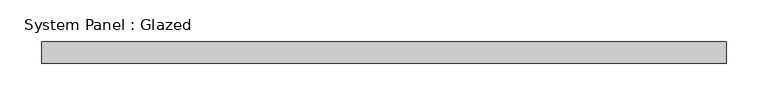
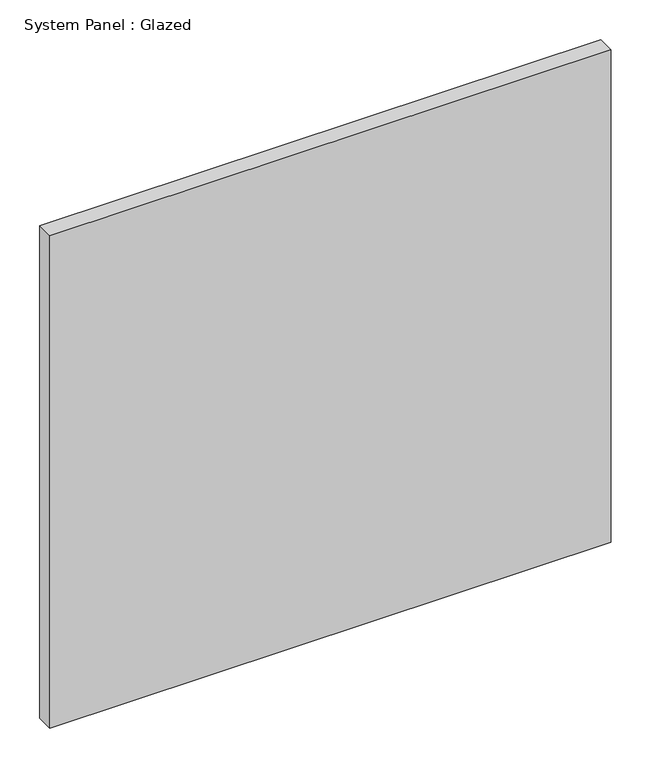
"""IFC4 building model written with IfcOpenShell, lengths in millimetres: plate geometry, System Panel : Glazed."""

from ifc_helpers import new_model, si_unit, origin, origin_with_axes, place, context, project, spatial, polyline, outline, extrude, source, transform, mapped, element, save


def system_panel_glazed_8adc4deb(model_context):
    return source(origin(), model_context, "Body", "SweptSolid", [
        extrude(outline(polyline([(409.575, 19.05), (-409.575, 19.05), (-409.575, 44.45), (409.575, 44.45), (409.575, 19.05)])), origin_with_axes(), (0.0, 0.0, 1.0), 759.593224),
    ])


if __name__ == "__main__":
    model = new_model("IFC4")
    model_context = context("Model", 3, world=origin())
    ifc_project = project(units=[si_unit("LENGTHUNIT", "METRE", prefix="MILLI")], contexts=[model_context])
    site = spatial("IfcSite", under=ifc_project)
    building = spatial("IfcBuilding", under=site)
    placement = place(None, origin())
    system_panel_glazed_shape = system_panel_glazed_8adc4deb(model_context)
    element("IfcPlate", 1, ObjectType="System Panel : Glazed", at=placement, inside=building, context=model_context, shape_type="MappedRepresentation", body=[
        mapped(system_panel_glazed_shape, transform((0.0, 0.0, 0.0), x_axis=(1.0, 0.0, 0.0), y_axis=(0.0, 1.0, 0.0), z_axis=(0.0, 0.0, 1.0))),
    ])
    save(model, "model.ifc")

# Revit data of these elements
# Type "System Panel : Glazed"
#   Construction Type Id = "GSP4R"
#   Analytic Construction = "1/8 in Pilkington single glazing"
#   Visual Light Transmittance = 0.9
#   Solar Heat Gain Coefficient = 0.86
#   Heat Transfer Coefficient (U) = 1.18115 BTU/(h·ft²·°F)
#   Define Thermal Properties by = 1
# Element 1 (IfcPlate, "System Panel : Glazed")
#   Materials on its faces: "Glass"
# Materials
#   "Glass": class "Glass", colour RGB 0 128 192, transparency 0.75, Description = "Soda Lime Glass", Cost = 0
